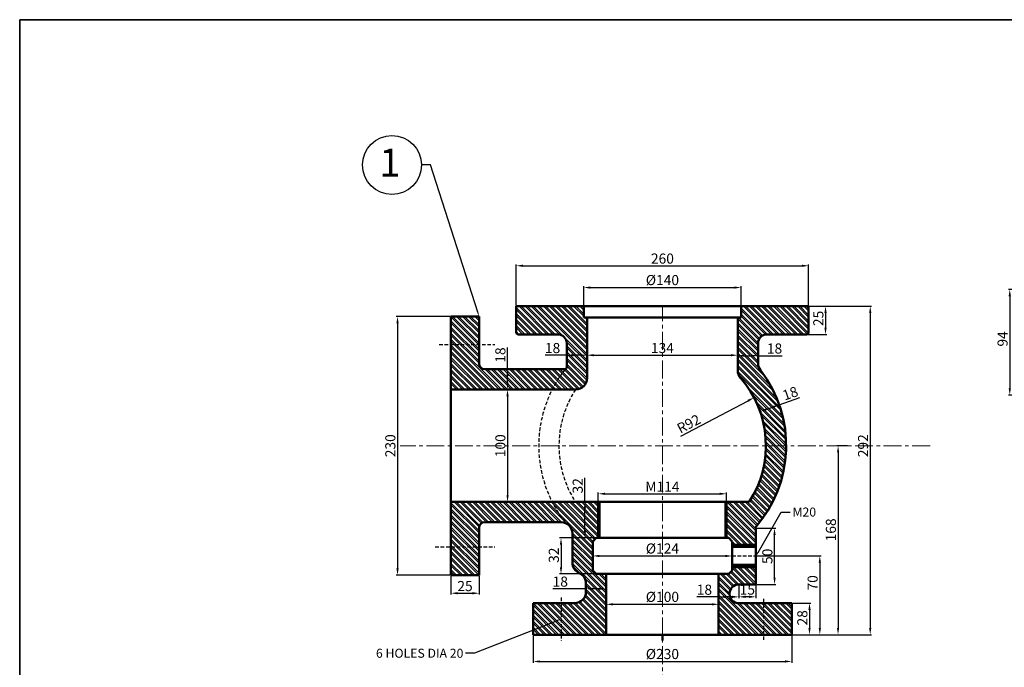
# Model space of a CAD drawing. Units: millimetres. Extents: x -282 to 2335, y -1129 to 664.
# Tile 3 of 8: x -282 to 594, y 88 to 664. Entities that reach past the tile are written whole.
import ezdxf
from ezdxf import colors
from ezdxf.entities.mleader import LeaderData, LeaderLine
from ezdxf.math import Vec2, Vec3

# ---------------------------------------------------------------- set-up
doc = ezdxf.new("R2010")
doc.units = ezdxf.units.MM
doc.header["$LTSCALE"] = 0.5
doc.linetypes.add('CENTER', pattern=[50.8, 31.75, -6.35, 6.35, -6.35])
doc.linetypes.add('HIDDEN', pattern=[9.525, 6.35, -3.175])
for name, color, linetype, lineweight in [('M-CNTR', 1, 'CENTER', 18), ('M-DIMS', 2, 'Continuous', 25), ('M-HATC', 8, 'Continuous', 18), ('M-HIDN', 4, 'HIDDEN', 25), ('M-OUTL', 7, 'Continuous', 50), ('M-TEXT', 3, 'Continuous', 25), ('M-TTLB', 7, 'Continuous', 35)]:
    doc.layers.add(name, color=color, linetype=linetype, lineweight=lineweight)
doc.styles.get("Standard").update_dxf_attribs({"font": 'arial.ttf'})
doc.dimstyles.new('ISO-25', dxfattribs={"dimtxt": 9, "dimasz": 6, "dimexe": 1.25, "dimexo": 0.625, "dimtad": 1, "dimtxsty": 'Standard', "dimcen": 2.5, "dimadec": 0, "dimazin": 0, "dimtfac": 1, "dimtofl": 0, "dimtmove": 0, "dimatfit": 3, "dimfxl": 1, "dimarcsym": 0})

# ---------------------------------------------------------------- blocks, each defined once
blk = doc.blocks.new('*D1')
at = {"layer": 'Defpoints', "color": 0, "transparency": 16777216}
for p in [(419.64, 444.96), (159.64, 408.91), (419.64, 408.91)]:
    blk.add_point(p, dxfattribs=at)
at = {"layer": 'M-DIMS', "color": 0, "lineweight": -2, "transparency": 16777216}
for p, q in [((159.64, 409.54), (159.64, 446.21)), ((165.64, 444.96), (413.64, 444.96)), ((419.64, 409.54), (419.64, 446.21))]:
    blk.add_line(p, q, dxfattribs=at)
at = {"layer": 'M-DIMS', "color": 0, "transparency": 16777216}
for points in [[(165.64, 445.96), (165.64, 443.96), (159.64, 444.96)], [(413.64, 445.96), (413.64, 443.96), (419.64, 444.96)]]:
    blk.add_solid(points, dxfattribs=at)
at = {"layer": 'M-DIMS', "color": 0, "transparency": 16777216, "insert": (289.64, 450.18), "char_height": 9, "attachment_point": 5}
blk.add_mtext('260', dxfattribs=at)
blk = doc.blocks.new('*D2')
at = {"layer": 'Defpoints', "color": 0, "transparency": 16777216}
for p in [(359.64, 425.58), (219.64, 408.91), (359.64, 408.91)]:
    blk.add_point(p, dxfattribs=at)
at = {"layer": 'M-DIMS', "color": 0, "lineweight": -2, "transparency": 16777216}
for p, q in [((219.64, 409.54), (219.64, 426.83)), ((225.64, 425.58), (353.64, 425.58)), ((359.64, 409.54), (359.64, 426.83))]:
    blk.add_line(p, q, dxfattribs=at)
at = {"layer": 'M-DIMS', "color": 0, "transparency": 16777216}
for points in [[(225.64, 426.58), (225.64, 424.58), (219.64, 425.58)], [(353.64, 426.58), (353.64, 424.58), (359.64, 425.58)]]:
    blk.add_solid(points, dxfattribs=at)
at = {"layer": 'M-DIMS', "color": 0, "transparency": 16777216, "insert": (289.64, 431.06), "char_height": 9, "attachment_point": 5}
blk.add_mtext('%%C140', dxfattribs=at)
blk = doc.blocks.new('*D3')
at = {"layer": 'Defpoints', "color": 0, "transparency": 16777216}
for p in [(101.64, 399.91), (54.14, 169.91), (101.64, 169.91)]:
    blk.add_point(p, dxfattribs=at)
at = {"layer": 'M-DIMS', "color": 0, "lineweight": -2, "transparency": 16777216}
for p, q in [((101.01, 399.91), (52.89, 399.91)), ((54.14, 393.91), (54.14, 175.91)), ((101.01, 169.91), (52.89, 169.91))]:
    blk.add_line(p, q, dxfattribs=at)
at = {"layer": 'M-DIMS', "color": 0, "transparency": 16777216}
for points in [[(53.14, 393.91), (55.14, 393.91), (54.14, 399.91)], [(53.14, 175.91), (55.14, 175.91), (54.14, 169.91)]]:
    blk.add_solid(points, dxfattribs=at)
at = {"layer": 'M-DIMS', "color": 0, "transparency": 16777216, "insert": (48.91, 284.91), "char_height": 9, "attachment_point": 5, "rotation": 90}
blk.add_mtext('230', dxfattribs=at)
blk = doc.blocks.new('*D4')
at = {"layer": 'Defpoints', "color": 0, "transparency": 16777216}
for p in [(157.14, 334.91), (151.94, 234.91), (157.14, 234.91)]:
    blk.add_point(p, dxfattribs=at)
at = {"layer": 'M-DIMS', "color": 0, "lineweight": -2, "transparency": 16777216}
for p, q in [((156.51, 334.91), (150.69, 334.91)), ((151.94, 328.91), (151.94, 240.91)), ((156.51, 234.91), (150.69, 234.91))]:
    blk.add_line(p, q, dxfattribs=at)
at = {"layer": 'M-DIMS', "color": 0, "transparency": 16777216}
for points in [[(150.94, 328.91), (152.94, 328.91), (151.94, 334.91)], [(150.94, 240.91), (152.94, 240.91), (151.94, 234.91)]]:
    blk.add_solid(points, dxfattribs=at)
at = {"layer": 'M-DIMS', "color": 0, "transparency": 16777216, "insert": (146.72, 284.91), "char_height": 9, "attachment_point": 5, "rotation": 90}
blk.add_mtext('100', dxfattribs=at)
blk = doc.blocks.new('*D5')
at = {"layer": 'Defpoints', "color": 0, "transparency": 16777216}
for p in [(151.94, 352.91), (151.94, 334.91), (151.94, 334.91)]:
    blk.add_point(p, dxfattribs=at)
at = {"layer": 'M-DIMS', "color": 0, "lineweight": -2, "transparency": 16777216}
for p, q in [((151.94, 352.91), (151.94, 372.22)), ((151.31, 352.91), (150.69, 352.91)), ((151.94, 340.91), (151.94, 346.91)), ((151.31, 334.91), (150.69, 334.91))]:
    blk.add_line(p, q, dxfattribs=at)
at = {"layer": 'M-DIMS', "color": 0, "transparency": 16777216}
for points in [[(150.94, 346.91), (152.94, 346.91), (151.94, 352.91)], [(150.94, 340.91), (152.94, 340.91), (151.94, 334.91)]]:
    blk.add_solid(points, dxfattribs=at)
at = {"layer": 'M-DIMS', "color": 0, "transparency": 16777216, "insert": (146.72, 365.57), "char_height": 9, "attachment_point": 5, "rotation": 90}
blk.add_mtext('18', dxfattribs=at)
blk = doc.blocks.new('*D6')
at = {"layer": 'Defpoints', "color": 0, "transparency": 16777216}
for p in [(204.64, 365.41), (222.64, 365.41), (222.64, 365.41)]:
    blk.add_point(p, dxfattribs=at)
at = {"layer": 'M-DIMS', "color": 0, "lineweight": -2, "transparency": 16777216}
for p, q in [((204.64, 365.41), (185.33, 365.41)), ((204.64, 366.04), (204.64, 366.66)), ((216.64, 365.41), (210.64, 365.41)), ((222.64, 366.04), (222.64, 366.66))]:
    blk.add_line(p, q, dxfattribs=at)
at = {"layer": 'M-DIMS', "color": 0, "transparency": 16777216}
for points in [[(210.64, 366.41), (210.64, 364.41), (204.64, 365.41)], [(216.64, 366.41), (216.64, 364.41), (222.64, 365.41)]]:
    blk.add_solid(points, dxfattribs=at)
at = {"layer": 'M-DIMS', "color": 0, "transparency": 16777216, "insert": (191.98, 370.63), "char_height": 9, "attachment_point": 5}
blk.add_mtext('18', dxfattribs=at)
blk = doc.blocks.new('*D7')
at = {"layer": 'Defpoints', "color": 0, "transparency": 16777216}
for p in [(222.64, 365.41), (356.64, 365.41), (356.64, 365.41)]:
    blk.add_point(p, dxfattribs=at)
at = {"layer": 'M-DIMS', "color": 0, "lineweight": -2, "transparency": 16777216}
for p, q in [((222.64, 366.04), (222.64, 366.66)), ((228.64, 365.41), (350.64, 365.41)), ((356.64, 366.04), (356.64, 366.66))]:
    blk.add_line(p, q, dxfattribs=at)
at = {"layer": 'M-DIMS', "color": 0, "transparency": 16777216}
for points in [[(228.64, 366.41), (228.64, 364.41), (222.64, 365.41)], [(350.64, 366.41), (350.64, 364.41), (356.64, 365.41)]]:
    blk.add_solid(points, dxfattribs=at)
at = {"layer": 'M-DIMS', "color": 0, "transparency": 16777216, "insert": (289.64, 370.63), "char_height": 9, "attachment_point": 5}
blk.add_mtext('134', dxfattribs=at)
blk = doc.blocks.new('*D8')
at = {"layer": 'Defpoints', "color": 0, "transparency": 16777216}
for p in [(234.25, 234.91), (220.71, 202.91), (234.25, 202.91)]:
    blk.add_point(p, dxfattribs=at)
at = {"layer": 'M-DIMS', "color": 0, "lineweight": -2, "transparency": 16777216}
for p, q in [((220.71, 234.91), (220.71, 256.3)), ((233.63, 234.91), (219.46, 234.91)), ((220.71, 208.91), (220.71, 228.91)), ((233.63, 202.91), (219.46, 202.91))]:
    blk.add_line(p, q, dxfattribs=at)
at = {"layer": 'M-DIMS', "color": 0, "transparency": 16777216}
for points in [[(219.71, 228.91), (221.71, 228.91), (220.71, 234.91)], [(219.71, 208.91), (221.71, 208.91), (220.71, 202.91)]]:
    blk.add_solid(points, dxfattribs=at)
at = {"layer": 'M-DIMS', "color": 0, "transparency": 16777216, "insert": (215.49, 249.28), "char_height": 9, "attachment_point": 5, "rotation": 90}
blk.add_mtext('32', dxfattribs=at)
blk = doc.blocks.new('*D9')
at = {"layer": 'Defpoints', "color": 0, "transparency": 16777216}
for p in [(101.64, 169.91), (126.64, 169.91), (126.64, 153.76)]:
    blk.add_point(p, dxfattribs=at)
at = {"layer": 'M-DIMS', "color": 0, "lineweight": -2, "transparency": 16777216}
for p, q in [((101.64, 169.29), (101.64, 152.51)), ((126.64, 169.29), (126.64, 152.51)), ((107.64, 153.76), (120.64, 153.76))]:
    blk.add_line(p, q, dxfattribs=at)
at = {"layer": 'M-DIMS', "color": 0, "transparency": 16777216}
for points in [[(107.64, 154.76), (107.64, 152.76), (101.64, 153.76)], [(120.64, 154.76), (120.64, 152.76), (126.64, 153.76)]]:
    blk.add_solid(points, dxfattribs=at)
at = {"layer": 'M-DIMS', "color": 0, "transparency": 16777216, "insert": (114.14, 158.98), "char_height": 9, "attachment_point": 5}
blk.add_mtext('25', dxfattribs=at)
blk = doc.blocks.new('*D10')
at = {"layer": 'Defpoints', "color": 0, "transparency": 16777216}
for p in [(174.64, 116.91), (404.64, 116.91), (404.64, 93.09)]:
    blk.add_point(p, dxfattribs=at)
at = {"layer": 'M-DIMS', "color": 0, "lineweight": -2, "transparency": 16777216}
for p, q in [((174.64, 116.29), (174.64, 91.84)), ((404.64, 116.29), (404.64, 91.84)), ((180.64, 93.09), (398.64, 93.09))]:
    blk.add_line(p, q, dxfattribs=at)
at = {"layer": 'M-DIMS', "color": 0, "transparency": 16777216}
for points in [[(180.64, 94.09), (180.64, 92.09), (174.64, 93.09)], [(398.64, 94.09), (398.64, 92.09), (404.64, 93.09)]]:
    blk.add_solid(points, dxfattribs=at)
at = {"layer": 'M-DIMS', "color": 0, "transparency": 16777216, "insert": (289.64, 98.56), "char_height": 9, "attachment_point": 5}
blk.add_mtext('%%C230', dxfattribs=at)
blk = doc.blocks.new('*D11')
at = {"layer": 'Defpoints', "color": 0, "transparency": 16777216}
for p in [(239.64, 143.91), (339.64, 143.91), (339.64, 143.91)]:
    blk.add_point(p, dxfattribs=at)
at = {"layer": 'M-DIMS', "color": 0, "lineweight": -2, "transparency": 16777216}
for p, q in [((239.64, 144.54), (239.64, 145.16)), ((245.64, 143.91), (333.64, 143.91)), ((339.64, 144.54), (339.64, 145.16))]:
    blk.add_line(p, q, dxfattribs=at)
at = {"layer": 'M-DIMS', "color": 0, "transparency": 16777216}
for points in [[(245.64, 144.91), (245.64, 142.91), (239.64, 143.91)], [(333.64, 144.91), (333.64, 142.91), (339.64, 143.91)]]:
    blk.add_solid(points, dxfattribs=at)
at = {"layer": 'M-DIMS', "color": 0, "transparency": 16777216, "insert": (289.64, 149.38), "char_height": 9, "attachment_point": 5}
blk.add_mtext('%%C100', dxfattribs=at)
blk = doc.blocks.new('*D12')
at = {"layer": 'Defpoints', "color": 0, "transparency": 16777216}
for p in [(227.64, 186.91), (351.64, 186.91), (351.64, 186.91)]:
    blk.add_point(p, dxfattribs=at)
at = {"layer": 'M-DIMS', "color": 0, "lineweight": -2, "transparency": 16777216}
for p, q in [((227.64, 187.54), (227.64, 188.16)), ((233.64, 186.91), (345.64, 186.91)), ((351.64, 187.54), (351.64, 188.16))]:
    blk.add_line(p, q, dxfattribs=at)
at = {"layer": 'M-DIMS', "color": 0, "transparency": 16777216}
for points in [[(233.64, 187.91), (233.64, 185.91), (227.64, 186.91)], [(345.64, 187.91), (345.64, 185.91), (351.64, 186.91)]]:
    blk.add_solid(points, dxfattribs=at)
at = {"layer": 'M-DIMS', "color": 0, "transparency": 16777216, "insert": (289.64, 192.38), "char_height": 9, "attachment_point": 5}
blk.add_mtext('%%C124', dxfattribs=at)
blk = doc.blocks.new('*D13')
at = {"layer": 'Defpoints', "color": 0, "transparency": 16777216}
for p in [(346.64, 242.19), (232.64, 234.91), (346.64, 234.91)]:
    blk.add_point(p, dxfattribs=at)
at = {"layer": 'M-DIMS', "color": 0, "lineweight": -2, "transparency": 16777216}
for p, q in [((232.64, 235.54), (232.64, 243.44)), ((238.64, 242.19), (340.64, 242.19)), ((346.64, 235.54), (346.64, 243.44))]:
    blk.add_line(p, q, dxfattribs=at)
at = {"layer": 'M-DIMS', "color": 0, "transparency": 16777216}
for points in [[(238.64, 243.19), (238.64, 241.19), (232.64, 242.19)], [(340.64, 243.19), (340.64, 241.19), (346.64, 242.19)]]:
    blk.add_solid(points, dxfattribs=at)
at = {"layer": 'M-DIMS', "color": 0, "transparency": 16777216, "insert": (289.64, 247.33), "char_height": 9, "attachment_point": 5}
blk.add_mtext('M114', dxfattribs=at)
blk = doc.blocks.new('*D14')
at = {"layer": 'Defpoints', "color": 0, "transparency": 16777216}
for p in [(234.25, 202.91), (199.48, 170.91), (234.25, 170.91)]:
    blk.add_point(p, dxfattribs=at)
at = {"layer": 'M-DIMS', "color": 0, "lineweight": -2, "transparency": 16777216}
for p, q in [((233.63, 202.91), (198.23, 202.91)), ((199.48, 196.91), (199.48, 176.91)), ((233.63, 170.91), (198.23, 170.91))]:
    blk.add_line(p, q, dxfattribs=at)
at = {"layer": 'M-DIMS', "color": 0, "transparency": 16777216}
for points in [[(198.48, 196.91), (200.48, 196.91), (199.48, 202.91)], [(198.48, 176.91), (200.48, 176.91), (199.48, 170.91)]]:
    blk.add_solid(points, dxfattribs=at)
at = {"layer": 'M-DIMS', "color": 0, "transparency": 16777216, "insert": (194.26, 187.54), "char_height": 9, "attachment_point": 5, "rotation": 90}
blk.add_mtext('32', dxfattribs=at)
blk = doc.blocks.new('*D15')
at = {"layer": 'Defpoints', "color": 0, "transparency": 16777216}
for p in [(221.64, 158.58), (221.64, 157.7), (239.64, 158.58)]:
    blk.add_point(p, dxfattribs=at)
at = {"layer": 'M-DIMS', "color": 0, "lineweight": -2, "transparency": 16777216}
for p, q in [((221.64, 157.7), (192.18, 157.7)), ((221.64, 157.95), (221.64, 156.45)), ((233.64, 157.7), (227.64, 157.7)), ((239.64, 157.95), (239.64, 156.45))]:
    blk.add_line(p, q, dxfattribs=at)
at = {"layer": 'M-DIMS', "color": 0, "transparency": 16777216}
for points in [[(227.64, 158.7), (227.64, 156.7), (221.64, 157.7)], [(233.64, 158.7), (233.64, 156.7), (239.64, 157.7)]]:
    blk.add_solid(points, dxfattribs=at)
at = {"layer": 'M-DIMS', "color": 0, "transparency": 16777216, "insert": (198.83, 162.92), "char_height": 9, "attachment_point": 5}
blk.add_mtext('18', dxfattribs=at)
blk = doc.blocks.new('*D16')
at = {"layer": 'Defpoints', "color": 0, "transparency": 16777216}
for p in [(404.64, 144.91), (404.64, 116.91), (420.41, 116.91)]:
    blk.add_point(p, dxfattribs=at)
at = {"layer": 'M-DIMS', "color": 0, "lineweight": -2, "transparency": 16777216}
for p, q in [((405.26, 144.91), (421.66, 144.91)), ((420.41, 138.91), (420.41, 122.91)), ((405.26, 116.91), (421.66, 116.91))]:
    blk.add_line(p, q, dxfattribs=at)
at = {"layer": 'M-DIMS', "color": 0, "transparency": 16777216}
for points in [[(419.41, 138.91), (421.41, 138.91), (420.41, 144.91)], [(419.41, 122.91), (421.41, 122.91), (420.41, 116.91)]]:
    blk.add_solid(points, dxfattribs=at)
at = {"layer": 'M-DIMS', "color": 0, "transparency": 16777216, "insert": (415.19, 131.9), "char_height": 9, "attachment_point": 5, "rotation": 90}
blk.add_mtext('28', dxfattribs=at)
blk = doc.blocks.new('*D17')
at = {"layer": 'Defpoints', "color": 0, "transparency": 16777216}
for p in [(372.64, 211.59), (389.33, 211.59), (372.64, 161.59)]:
    blk.add_point(p, dxfattribs=at)
at = {"layer": 'M-DIMS', "color": 0, "lineweight": -2, "transparency": 16777216}
for p, q in [((373.26, 211.59), (390.58, 211.59)), ((389.33, 167.59), (389.33, 205.59)), ((373.26, 161.59), (390.58, 161.59))]:
    blk.add_line(p, q, dxfattribs=at)
at = {"layer": 'M-DIMS', "color": 0, "transparency": 16777216}
for points in [[(388.33, 205.59), (390.33, 205.59), (389.33, 211.59)], [(388.33, 167.59), (390.33, 167.59), (389.33, 161.59)]]:
    blk.add_solid(points, dxfattribs=at)
at = {"layer": 'M-DIMS', "color": 0, "transparency": 16777216, "insert": (384.11, 186.58), "char_height": 9, "attachment_point": 5, "rotation": 90}
blk.add_mtext('50', dxfattribs=at)
blk = doc.blocks.new('*D18')
at = {"layer": 'Defpoints', "color": 0, "transparency": 16777216}
for p in [(339.64, 152.65), (357.64, 153.25), (357.64, 150.54)]:
    blk.add_point(p, dxfattribs=at)
at = {"layer": 'M-DIMS', "color": 0, "lineweight": -2, "transparency": 16777216}
for p, q in [((339.64, 150.54), (320.33, 150.54)), ((339.64, 152.02), (339.64, 149.29)), ((351.64, 150.54), (345.64, 150.54)), ((357.64, 152.63), (357.64, 149.29))]:
    blk.add_line(p, q, dxfattribs=at)
at = {"layer": 'M-DIMS', "color": 0, "transparency": 16777216}
for points in [[(345.64, 151.54), (345.64, 149.54), (339.64, 150.54)], [(351.64, 151.54), (351.64, 149.54), (357.64, 150.54)]]:
    blk.add_solid(points, dxfattribs=at)
at = {"layer": 'M-DIMS', "color": 0, "transparency": 16777216, "insert": (326.98, 155.76), "char_height": 9, "attachment_point": 5}
blk.add_mtext('18', dxfattribs=at)
blk = doc.blocks.new('*D19')
at = {"layer": 'Defpoints', "color": 0, "transparency": 16777216}
for p in [(357.64, 161.59), (372.64, 161.59), (357.64, 150.58)]:
    blk.add_point(p, dxfattribs=at)
at = {"layer": 'M-DIMS', "color": 0, "lineweight": -2, "transparency": 16777216}
for p, q in [((357.64, 160.96), (357.64, 149.33)), ((372.64, 160.96), (372.64, 149.33)), ((366.64, 150.58), (363.64, 150.58))]:
    blk.add_line(p, q, dxfattribs=at)
at = {"layer": 'M-DIMS', "color": 0, "transparency": 16777216}
for points in [[(363.64, 151.58), (363.64, 149.58), (357.64, 150.58)], [(366.64, 151.58), (366.64, 149.58), (372.64, 150.58)]]:
    blk.add_solid(points, dxfattribs=at)
at = {"layer": 'M-DIMS', "color": 0, "transparency": 16777216, "insert": (365.14, 155.8), "char_height": 9, "attachment_point": 5}
blk.add_mtext('15', dxfattribs=at)
blk = doc.blocks.new('*D20')
at = {"layer": 'Defpoints', "color": 0, "transparency": 16777216}
for p in [(372.64, 186.91), (382.34, 116.91), (429.57, 116.91)]:
    blk.add_point(p, dxfattribs=at)
at = {"layer": 'M-DIMS', "color": 0, "lineweight": -2, "transparency": 16777216}
for p, q in [((373.26, 186.91), (430.82, 186.91)), ((429.57, 180.91), (429.57, 122.91)), ((382.97, 116.91), (430.82, 116.91))]:
    blk.add_line(p, q, dxfattribs=at)
at = {"layer": 'M-DIMS', "color": 0, "transparency": 16777216}
for points in [[(428.57, 180.91), (430.57, 180.91), (429.57, 186.91)], [(428.57, 122.91), (430.57, 122.91), (429.57, 116.91)]]:
    blk.add_solid(points, dxfattribs=at)
at = {"layer": 'M-DIMS', "color": 0, "transparency": 16777216, "insert": (424.35, 163.01), "char_height": 9, "attachment_point": 5, "rotation": 90}
blk.add_mtext('70', dxfattribs=at)
blk = doc.blocks.new('*D21')
at = {"layer": 'Defpoints', "color": 0, "transparency": 16777216}
for p in [(454.95, 284.91), (404.64, 116.91), (445.81, 116.91)]:
    blk.add_point(p, dxfattribs=at)
at = {"layer": 'M-DIMS', "color": 0, "lineweight": -2, "transparency": 16777216}
for p, q in [((454.32, 284.91), (444.56, 284.91)), ((445.81, 278.91), (445.81, 122.91)), ((405.26, 116.91), (447.06, 116.91))]:
    blk.add_line(p, q, dxfattribs=at)
at = {"layer": 'M-DIMS', "color": 0, "transparency": 16777216}
for points in [[(444.81, 278.91), (446.81, 278.91), (445.81, 284.91)], [(444.81, 122.91), (446.81, 122.91), (445.81, 116.91)]]:
    blk.add_solid(points, dxfattribs=at)
at = {"layer": 'M-DIMS', "color": 0, "transparency": 16777216, "insert": (440.59, 210.12), "char_height": 9, "attachment_point": 5, "rotation": 90}
blk.add_mtext('168', dxfattribs=at)
blk = doc.blocks.new('*D22')
at = {"layer": 'Defpoints', "color": 0, "transparency": 16777216}
for p in [(359.64, 408.91), (359.64, 116.91), (474.41, 116.91)]:
    blk.add_point(p, dxfattribs=at)
at = {"layer": 'M-DIMS', "color": 0, "lineweight": -2, "transparency": 16777216}
for p, q in [((360.26, 408.91), (475.66, 408.91)), ((474.41, 402.91), (474.41, 122.91)), ((360.26, 116.91), (475.66, 116.91))]:
    blk.add_line(p, q, dxfattribs=at)
at = {"layer": 'M-DIMS', "color": 0, "transparency": 16777216}
for points in [[(473.41, 402.91), (475.41, 402.91), (474.41, 408.91)], [(473.41, 122.91), (475.41, 122.91), (474.41, 116.91)]]:
    blk.add_solid(points, dxfattribs=at)
at = {"layer": 'M-DIMS', "color": 0, "transparency": 16777216, "insert": (469.19, 284.91), "char_height": 9, "attachment_point": 5, "rotation": 90}
blk.add_mtext('292', dxfattribs=at)
blk = doc.blocks.new('*D23')
at = {"layer": 'Defpoints', "color": 0, "transparency": 16777216}
for p in [(371.08, 327.71), (289.64, 284.91)]:
    blk.add_point(p, dxfattribs=at)
at = {"layer": 'M-DIMS', "color": 0, "lineweight": -2, "transparency": 16777216}
blk.add_line((305.96, 293.49), (365.77, 324.91), dxfattribs=at)
at = {"layer": 'M-DIMS', "color": 0, "transparency": 16777216}
blk.add_solid([(365.3, 325.8), (366.23, 324.03), (371.08, 327.71)], dxfattribs=at)
at = {"layer": 'M-DIMS', "color": 0, "transparency": 16777216, "insert": (313.56, 303.38), "char_height": 9, "attachment_point": 5, "rotation": 27.72024}
blk.add_mtext('R92', dxfattribs=at)
blk = doc.blocks.new('*D24')
at = {"layer": 'Defpoints', "color": 0, "transparency": 16777216}
for p in [(376.46, 315.35), (393.44, 321.3), (393.44, 321.3)]:
    blk.add_point(p, dxfattribs=at)
at = {"layer": 'M-DIMS', "color": 0, "lineweight": -2, "transparency": 16777216}
for p, q in [((393.44, 321.3), (411.67, 327.69)), ((382.12, 317.33), (387.78, 319.32)), ((393.65, 320.71), (393.86, 320.12)), ((376.67, 314.76), (376.87, 314.17))]:
    blk.add_line(p, q, dxfattribs=at)
at = {"layer": 'M-DIMS', "color": 0, "transparency": 16777216}
for points in [[(381.79, 318.28), (382.45, 316.39), (376.46, 315.35)], [(387.45, 320.26), (388.11, 318.37), (393.44, 321.3)]]:
    blk.add_solid(points, dxfattribs=at)
at = {"layer": 'M-DIMS', "color": 0, "transparency": 16777216, "insert": (403.66, 330.42), "char_height": 9, "attachment_point": 5, "rotation": 19.31887}
blk.add_mtext('18', dxfattribs=at)
blk = doc.blocks.new('*D25')
at = {"layer": 'Defpoints', "color": 0, "transparency": 16777216}
for p in [(419.64, 408.91), (413.92, 383.91), (434.65, 383.91)]:
    blk.add_point(p, dxfattribs=at)
at = {"layer": 'M-DIMS', "color": 0, "lineweight": -2, "transparency": 16777216}
for p, q in [((420.26, 408.91), (435.9, 408.91)), ((434.65, 402.91), (434.65, 389.91)), ((414.54, 383.91), (435.9, 383.91))]:
    blk.add_line(p, q, dxfattribs=at)
at = {"layer": 'M-DIMS', "color": 0, "transparency": 16777216}
for points in [[(433.65, 402.91), (435.65, 402.91), (434.65, 408.91)], [(433.65, 389.91), (435.65, 389.91), (434.65, 383.91)]]:
    blk.add_solid(points, dxfattribs=at)
at = {"layer": 'M-DIMS', "color": 0, "transparency": 16777216, "insert": (429.43, 398.14), "char_height": 9, "attachment_point": 5, "rotation": 90}
blk.add_mtext('25', dxfattribs=at)
blk = doc.blocks.new('*D26')
at = {"layer": 'Defpoints', "color": 0, "transparency": 16777216}
for p in [(356.64, 365.41), (374.64, 365.41), (374.64, 364.99)]:
    blk.add_point(p, dxfattribs=at)
at = {"layer": 'M-DIMS', "color": 0, "lineweight": -2, "transparency": 16777216}
for p, q in [((356.64, 364.79), (356.64, 363.74)), ((362.64, 364.99), (368.64, 364.99)), ((374.64, 364.99), (395.97, 364.99)), ((374.64, 364.79), (374.64, 363.74))]:
    blk.add_line(p, q, dxfattribs=at)
at = {"layer": 'M-DIMS', "color": 0, "transparency": 16777216}
for points in [[(362.64, 365.99), (362.64, 363.99), (356.64, 364.99)], [(368.64, 365.99), (368.64, 363.99), (374.64, 364.99)]]:
    blk.add_solid(points, dxfattribs=at)
at = {"layer": 'M-DIMS', "color": 0, "transparency": 16777216, "insert": (389.31, 370.21), "char_height": 9, "attachment_point": 5}
blk.add_mtext('18', dxfattribs=at)
blk = doc.blocks.new('*D29')
at = {"layer": 'Defpoints', "color": 0, "transparency": 16777216}
for p in [(289.64, 408.91), (438.52, 1.98), (289.64, -83.98), (321.01, -89.51), (289.64, -321.19)]:
    blk.add_point(p, dxfattribs=at)
at = {"layer": 'M-DIMS', "color": 0, "lineweight": -2, "transparency": 16777216}
blk.add_arc((289.64, -83.98), 31.85, 280.80805, 19.19195, dxfattribs=at)
at = {"layer": 'M-DIMS', "color": 0, "transparency": 16777216}
for points in [[(318.81, -73.92), (320.63, -73.09), (317.23, -68.05)], [(295.71, -116.26), (295.52, -114.27), (289.64, -115.83)]]:
    blk.add_solid(points, dxfattribs=at)
at = {"layer": 'M-DIMS', "color": 0, "transparency": 16777216, "insert": (311.25, -99.54), "char_height": 9, "attachment_point": 5, "rotation": 54.2496}
blk.add_mtext('120°', dxfattribs=at)
blk = doc.blocks.new('*D31')
at = {"layer": 'Defpoints', "color": 0, "transparency": 16777216}
for p in [(645.29, 423.91), (598.46, 329.91), (615.29, 329.91)]:
    blk.add_point(p, dxfattribs=at)
at = {"layer": 'M-DIMS', "color": 0, "lineweight": -2, "transparency": 16777216}
for p, q in [((644.66, 423.91), (597.21, 423.91)), ((598.46, 417.91), (598.46, 335.91)), ((614.66, 329.91), (597.21, 329.91))]:
    blk.add_line(p, q, dxfattribs=at)
at = {"layer": 'M-DIMS', "color": 0, "transparency": 16777216}
for points in [[(597.46, 417.91), (599.46, 417.91), (598.46, 423.91)], [(597.46, 335.91), (599.46, 335.91), (598.46, 329.91)]]:
    blk.add_solid(points, dxfattribs=at)
at = {"layer": 'M-DIMS', "color": 0, "transparency": 16777216, "insert": (593.24, 379.91), "char_height": 9, "attachment_point": 5, "rotation": 90}
blk.add_mtext('94', dxfattribs=at)

msp = doc.modelspace()

# ---------------------------------------------------------------- hatches: boundary and pattern name
at = {"layer": 'M-HATC'}
h = msp.add_hatch(dxfattribs=at)
h.set_pattern_fill('ANSI32', color=256, scale=0.4, angle=90)
h.paths.add_polyline_path([(376.722, 352.116, -0.165811), (374.639, 358.225), (374.639, 375.911, -0.4142136), (382.639, 383.911), (417.639, 383.911, 0.4142136), (419.639, 385.911), (419.639, 408.911), (359.639, 408.911), (359.639, 398.911), (356.639, 398.911), (356.639, 351.806, 0.1807537), (359.09, 345.248, -0.1807537), (381.639, 284.911), (399.639, 284.911, 0.165811)])
h.paths.add_polyline_path([(399.639, 284.911), (381.639, 284.911, -0.14464), (366.866, 234.911), (346.639, 234.911), (346.639, 202.911), (348.639, 202.911), (351.639, 199.911), (351.639, 196.911), (372.639, 196.911), (372.639, 211.59), (371.978, 211.971, 0.1832453)])
h.paths.add_polyline_path([(372.639, 176.911), (351.639, 176.911), (351.639, 173.911), (348.639, 170.911), (339.639, 170.911), (339.639, 116.911), (404.639, 116.911), (404.639, 144.911), (357.639, 144.911, -1), (357.639, 161.59), (372.639, 161.59)])
h.paths.add_polyline_path([(239.639, 170.911), (230.639, 170.911), (227.639, 173.911), (227.639, 199.911), (230.639, 202.911), (232.639, 202.911), (232.639, 234.911), (191.659, 234.911, 0.0515301), (203.954, 215.932, -0.28881), (209.639, 206.911), (209.639, 180.911, 0.2982166), (215.639, 171.746, -0.2982166), (221.639, 162.581), (221.639, 154.911, -0.4142136), (211.639, 144.911), (174.639, 144.911), (174.639, 116.911), (239.639, 116.911)])
h.paths.add_polyline_path([(191.659, 234.911), (101.639, 234.911), (101.639, 194.911), (126.639, 194.911), (126.639, 211.911, -0.4142136), (131.639, 216.911), (199.639, 216.911, -0.1120046), (203.954, 215.932, -0.0515301)])
h.paths.add_polyline_path([(126.639, 194.911), (101.639, 194.911), (101.639, 169.911), (126.639, 169.911)])
h.paths.add_polyline_path([(203.25, 353.007, -0.077846), (202.639, 352.911), (131.639, 352.911, -0.4142136), (126.639, 357.911), (126.639, 374.911), (101.639, 374.911), (101.639, 334.911), (191.659, 334.911, -0.0489576)])
h.paths.add_polyline_path([(126.639, 399.911), (101.639, 399.911), (101.639, 374.911), (126.639, 374.911)])
h.paths.add_polyline_path([(222.639, 398.911), (219.639, 398.911), (219.639, 408.911), (159.639, 408.911), (159.639, 385.911, 0.4142136), (161.639, 383.911), (196.639, 383.911, -0.4142136), (204.639, 375.911), (204.639, 354.911, -0.3258602), (203.25, 353.007, 0.0489576), (191.659, 334.911), (212.639, 334.911, 0.4142136), (222.639, 344.911)])

# ---------------------------------------------------------------- linework, layer by layer
at = {"layer": 'M-CNTR'}
for p, q in [((289.639, -213.977), (289.639, 408.911)), ((527.55, 284.911), (56.464, 284.911))]:
    msp.add_line(p, q, dxfattribs=at)
at = {"layer": 'M-HIDN'}
for p, q in [((91.146, 374.911), (140.735, 374.911)), ((87.713, 194.911), (140.735, 194.911)), ((351.639, 186.911), (372.639, 186.911)), ((199.639, 150.014), (199.639, 111.673)), ((379.639, 148.714), (379.639, 111.673))]:
    msp.add_line(p, q, dxfattribs=at)
for radius, start, end in [(110, 141.816518, 218.835076), (92, 147.079265, 212.920735)]:
    msp.add_arc((289.639, 284.911), radius, start, end, dxfattribs=at)
at = {"layer": 'M-OUTL'}
for p, q in [((219.639, 408.911), (159.639, 408.911)), ((159.639, 408.911), (159.639, 385.911)), ((219.639, 408.911), (359.639, 408.911)), ((219.639, 398.911), (219.639, 408.911)), ((359.639, 408.911), (359.639, 398.911)), ((359.639, 408.911), (419.639, 408.911)), ((419.639, 408.911), (419.639, 385.911)), ((101.639, 169.911), (101.639, 399.911)), ((101.639, 399.911), (126.639, 399.911)), ((126.639, 399.911), (126.639, 357.911)), ((359.639, 398.911), (219.639, 398.911)), ((222.639, 398.911), (222.639, 344.911)), ((356.639, 398.911), (356.639, 351.806)), ((161.639, 383.911), (196.639, 383.911)), ((417.639, 383.911), (382.639, 383.911)), ((204.639, 375.911), (204.639, 354.911)), ((374.639, 375.911), (374.639, 358.225)), ((202.639, 352.911), (131.639, 352.911)), ((212.639, 334.911), (101.639, 334.911)), ((366.639, 334.911), (366.866, 334.911)), ((366.866, 234.911), (101.639, 234.911)), ((232.639, 234.911), (232.639, 202.911)), ((233.639, 234.911), (233.639, 202.911)), ((345.639, 234.911), (345.639, 202.911)), ((346.639, 234.911), (346.639, 202.911)), ((126.639, 211.911), (126.639, 169.911)), ((199.639, 216.911), (131.639, 216.911)), ((372.639, 211.59), (371.978, 211.971)), ((372.639, 165.343), (372.639, 211.59)), ((372.639, 211.59), (372.639, 161.59)), ((209.639, 206.911), (209.639, 180.911)), ((230.639, 202.911), (227.639, 199.911)), ((230.639, 202.911), (348.639, 202.911)), ((348.639, 202.911), (351.639, 199.911)), ((227.639, 199.911), (227.639, 173.911)), ((351.639, 173.911), (351.639, 199.911)), ((351.639, 196.911), (372.639, 196.911)), ((351.639, 194.911), (372.639, 194.911)), ((351.639, 178.911), (372.639, 178.911)), ((351.639, 176.911), (372.639, 176.911)), ((126.639, 169.911), (101.639, 169.911)), ((227.639, 173.911), (230.639, 170.911)), ((230.639, 170.911), (348.639, 170.911)), ((239.639, 170.911), (239.639, 116.911)), ((339.639, 170.911), (339.639, 116.911)), ((351.639, 173.911), (348.639, 170.911)), ((221.639, 162.581), (221.639, 154.911)), ((372.639, 161.59), (357.639, 161.59)), ((174.639, 144.911), (174.639, 116.911)), ((211.639, 144.911), (174.639, 144.911)), ((404.639, 144.911), (357.639, 144.911)), ((404.639, 116.911), (404.639, 144.911)), ((174.639, 116.911), (404.639, 116.911)), ((289.639, 116.911), (289.639, 111.673))]:
    msp.add_line(p, q, dxfattribs=at)
for centre, radius, start, end in [((161.639, 385.911), 2, 180, 270), ((417.639, 385.911), 2, 270, 0), ((196.639, 375.911), 8, 0, 90), ((382.639, 375.911), 8, 90, 180), ((131.639, 357.911), 5, 180, 270), ((202.639, 354.911), 2, 270, 0), ((366.639, 351.806), 10, 180, 220.983196), ((289.639, 284.911), 110, 318.464087, 37.658462), ((384.639, 358.225), 10, 180, 217.658462), ((212.639, 344.911), 10, 270, 0), ((289.639, 284.911), 92, 327.079265, 40.983196), ((131.639, 211.911), 5, 90, 180), ((199.639, 206.911), 10, 0, 90), ((219.639, 180.911), 10, 180, 246.421822), ((211.639, 162.581), 10, 0, 66.421822), ((357.639, 153.25), 8.339, 90, 270), ((211.639, 154.911), 10, 270, 0)]:
    msp.add_arc(centre, radius, start, end, dxfattribs=at)
at = {"layer": 'M-TEXT'}
msp.add_circle((49.217, 534.582), 26.287, dxfattribs=at)
at = {"layer": 'M-TTLB', "ltscale": 0.5}
msp.add_lwpolyline([(-281.776, 663.767), (2334.915, 663.767), (2334.915, -1128.523), (-281.776, -1128.523)], close=True, dxfattribs=at)

# ---------------------------------------------------------------- texts
at = {"layer": 'M-TEXT', "insert": (34.883, 549.122), "char_height": 25, "attachment_point": 1}
msp.add_mtext_dynamic_manual_height_columns('\\pxqc;1', width=25, gutter_width=12.5, heights=[7.196], dxfattribs=at)

# ---------------------------------------------------------------- dimensions: what is measured, and where the dimension line sits
at = {"layer": 'M-DIMS'}
dim = msp.add_linear_dim(base=(419.639, 444.96), p1=(159.639, 408.911), p2=(419.639, 408.911), dimstyle='ISO-25', override={"dimclrd": 0, "dimclre": 0, "dimclrt": 0}, dxfattribs=at)
dim.commit()
dim.dimension.update_dxf_attribs({"geometry": '*D1', "text_midpoint": (289.639, 450.18)})
dim = msp.add_linear_dim(base=(359.639, 425.584), p1=(219.639, 408.911), p2=(359.639, 408.911), text='%%C<>', dimstyle='ISO-25', override={"dimclrd": 0, "dimclre": 0, "dimclrt": 0}, dxfattribs=at)
dim.commit()
dim.dimension.update_dxf_attribs({"geometry": '*D2', "text_midpoint": (289.639, 431.056)})
for base, p1, p2, angle, picture, middle, dimtype in [((598.463, 329.912), (645.287, 423.912), (615.287, 329.912), 90, '*D31', (598.463, 379.912), 160), ((474.406, 116.911), (359.639, 408.911), (359.639, 116.911), 90, '*D22', (474.406, 284.911), 160), ((434.649, 383.911), (419.639, 408.911), (413.915, 383.911), 90, '*D25', (434.649, 398.138), 160), ((151.938, 334.911), (151.938, 352.911), (151.938, 334.911), 90, '*D5', (151.938, 365.568), 160), ((393.445, 321.302), (376.458, 315.347), (393.445, 321.302), 19.31887, '*D24', (405.389, 325.489), 161), ((445.81, 116.911), (454.948, 284.911), (404.639, 116.911), 90, '*D21', (445.81, 210.115), 160), ((220.709, 202.911), (234.252, 234.911), (234.252, 202.911), 90, '*D8', (220.709, 249.283), 160), ((389.333, 211.59), (372.639, 161.59), (372.639, 211.59), 90, '*D17', (389.333, 186.575), 160), ((199.484, 170.911), (234.252, 202.911), (234.252, 170.911), 90, '*D14', (199.484, 187.542), 160), ((429.569, 116.911), (372.639, 186.911), (382.343, 116.911), 90, '*D20', (429.569, 163.011), 160), ((420.413, 116.911), (404.639, 144.911), (404.639, 116.911), 90, '*D16', (420.413, 131.899), 160)]:
    dim = msp.add_linear_dim(base=base, p1=p1, p2=p2, angle=angle, dimstyle='ISO-25', override={"dimclrd": 0, "dimclre": 0, "dimclrt": 0}, dxfattribs=at)
    dim.commit()
    dim.dimension.update_dxf_attribs({"geometry": picture, "text_midpoint": middle, "dimtype": dimtype})
dim = msp.add_angular_dim_2l(base=(321.009, -89.508), line1=((289.639, -83.977), (438.52, 1.98)), line2=((289.639, -321.193), (289.639, 408.911)), dimstyle='ISO-25', override={"dimclrd": 0, "dimclre": 0, "dimclrt": 0}, dxfattribs=at)
dim.commit()
dim.dimension.update_dxf_attribs({"geometry": '*D29', "text_midpoint": (315.491, -102.588), "dimtype": 162})
for base, p1, p2, picture, middle in [((54.137, 169.911), (101.639, 399.911), (101.639, 169.911), '*D3', (48.914, 284.911)), ((151.938, 234.911), (157.139, 334.911), (157.139, 234.911), '*D4', (146.718, 284.911))]:
    dim = msp.add_linear_dim(base=base, p1=p1, p2=p2, angle=90, dimstyle='ISO-25', override={"dimclrd": 0, "dimclre": 0, "dimclrt": 0}, dxfattribs=at)
    dim.commit()
    dim.dimension.update_dxf_attribs({"geometry": picture, "text_midpoint": middle})
for base, p1, p2, picture, middle in [((222.639, 365.411), (204.639, 365.411), (222.639, 365.411), '*D6', (191.982, 365.411)), ((356.639, 365.411), (222.639, 365.411), (356.639, 365.411), '*D7', (289.639, 365.411)), ((374.639, 364.988), (356.639, 365.411), (374.639, 365.411), '*D26', (389.311, 364.988)), ((126.639, 153.756), (101.639, 169.911), (126.639, 169.911), '*D9', (114.139, 153.756)), ((221.639, 157.699), (239.639, 158.576), (221.639, 158.576), '*D15', (198.834, 157.699)), ((357.639, 150.541), (339.639, 152.647), (357.639, 153.25), '*D18', (326.982, 150.541)), ((357.639, 150.58), (372.639, 161.59), (357.639, 161.59), '*D19', (365.139, 150.58))]:
    dim = msp.add_linear_dim(base=base, p1=p1, p2=p2, dimstyle='ISO-25', override={"dimclrd": 0, "dimclre": 0, "dimclrt": 0}, dxfattribs=at)
    dim.commit()
    dim.dimension.update_dxf_attribs({"geometry": picture, "text_midpoint": middle, "dimtype": 160})
dim = msp.add_radius_dim(center=(289.639, 284.911), mpoint=(371.08, 327.705), dimstyle='ISO-25', override={"dimclrd": 0, "dimclre": 0, "dimclrt": 0}, dxfattribs=at)
dim.commit()
dim.dimension.update_dxf_attribs({"geometry": '*D23', "text_midpoint": (315.991, 298.758), "dimtype": 164})
for base, p1, p2, text, picture, middle in [((346.639, 242.188), (232.639, 234.911), (346.639, 234.911), 'M<>', '*D13', (289.639, 242.188)), ((351.639, 186.911), (227.639, 186.911), (351.639, 186.911), '%%C<>', '*D12', (289.639, 186.911)), ((339.639, 143.911), (239.639, 143.911), (339.639, 143.911), '%%C<>', '*D11', (289.639, 143.911)), ((404.639, 93.088), (174.639, 116.911), (404.639, 116.911), '%%C<>', '*D10', (289.639, 93.088))]:
    dim = msp.add_linear_dim(base=base, p1=p1, p2=p2, text=text, dimstyle='ISO-25', override={"dimclrd": 0, "dimclre": 0, "dimclrt": 0}, dxfattribs=at)
    dim.commit()
    dim.dimension.update_dxf_attribs({"geometry": picture, "text_midpoint": middle, "dimtype": 160})

# ---------------------------------------------------------------- leaders
at = {"layer": 'M-TEXT', "ltscale": 0.5}
ml = msp.add_multileader_mtext('Standard', dxfattribs=at)
ml.set_content('', color=256)
ml.set_leader_properties()
ml.build(insert=Vec2(0, 0))
ctx = ml.context
ctx.base_point, ctx.plane_origin = Vec3(71.503, 534.582), Vec3(126.639, 399.911)
ctx.text_align_type = 2
notes = []
notes.append((ctx, [(0, (1, 1, 0), (83.503, 534.582), (-1, 0), 8, [(0, [(126.639, 399.911)], 0, [])])]))
ctx.mtext.insert, ctx.mtext.alignment, ctx.mtext.flow_direction = Vec3(73.503, 536.582), 3, 5
at = {"layer": 'M-TEXT'}
ml = msp.add_multileader_mtext('Standard', dxfattribs=at)
ml.set_content('M20', color=256)
ml.set_leader_properties()
ml.build(insert=Vec2(0, 0))
ctx = ml.context
ctx.base_point, ctx.char_height, ctx.plane_origin = Vec3(403.321, 225.877), 8, Vec3(372.639, 186.59)
notes.append((ctx, [(0, (1, 1, 0), (395.321, 225.877), (1, 0), 8, [(0, [(372.639, 186.59)], 0, [])])]))
ctx.mtext.insert, ctx.mtext.flow_direction = Vec3(405.321, 229.945), 5
ml = msp.add_multileader_mtext('Standard', dxfattribs=at)
ml.set_content('6 HOLES DIA 20', color=256)
ml.set_leader_properties()
ml.build(insert=Vec2(0, 0))
ctx = ml.context
ctx.base_point, ctx.char_height, ctx.plane_origin = Vec3(27.18, 100.339), 8, Vec3(199.639, 130.844)
ctx.text_align_type = 2
notes.append((ctx, [(0, (1, 1, 0), (122.706, 100.339), (-1, 0), 8, [(0, [(199.639, 130.844)], 0, [])])]))
ctx.mtext.insert, ctx.mtext.alignment, ctx.mtext.flow_direction = Vec3(112.706, 104.407), 3, 5
for ctx, leaders in notes:
    for number, flags, end, landing, length, lines in leaders:
        leader = LeaderData()
        leader.index, (leader.has_last_leader_line, leader.has_dogleg_vector, leader.attachment_direction) = number, flags
        leader.last_leader_point, leader.dogleg_vector, leader.dogleg_length = Vec3(end), Vec3(landing), length
        for number, points, colour, breaks in lines:
            line = LeaderLine()
            line.index, line.vertices, line.color, line.breaks = number, Vec3.list(points), colors.encode_raw_color(colour), breaks
            leader.lines.append(line)
        ctx.leaders.append(leader)

doc.saveas('drawing.dxf')
